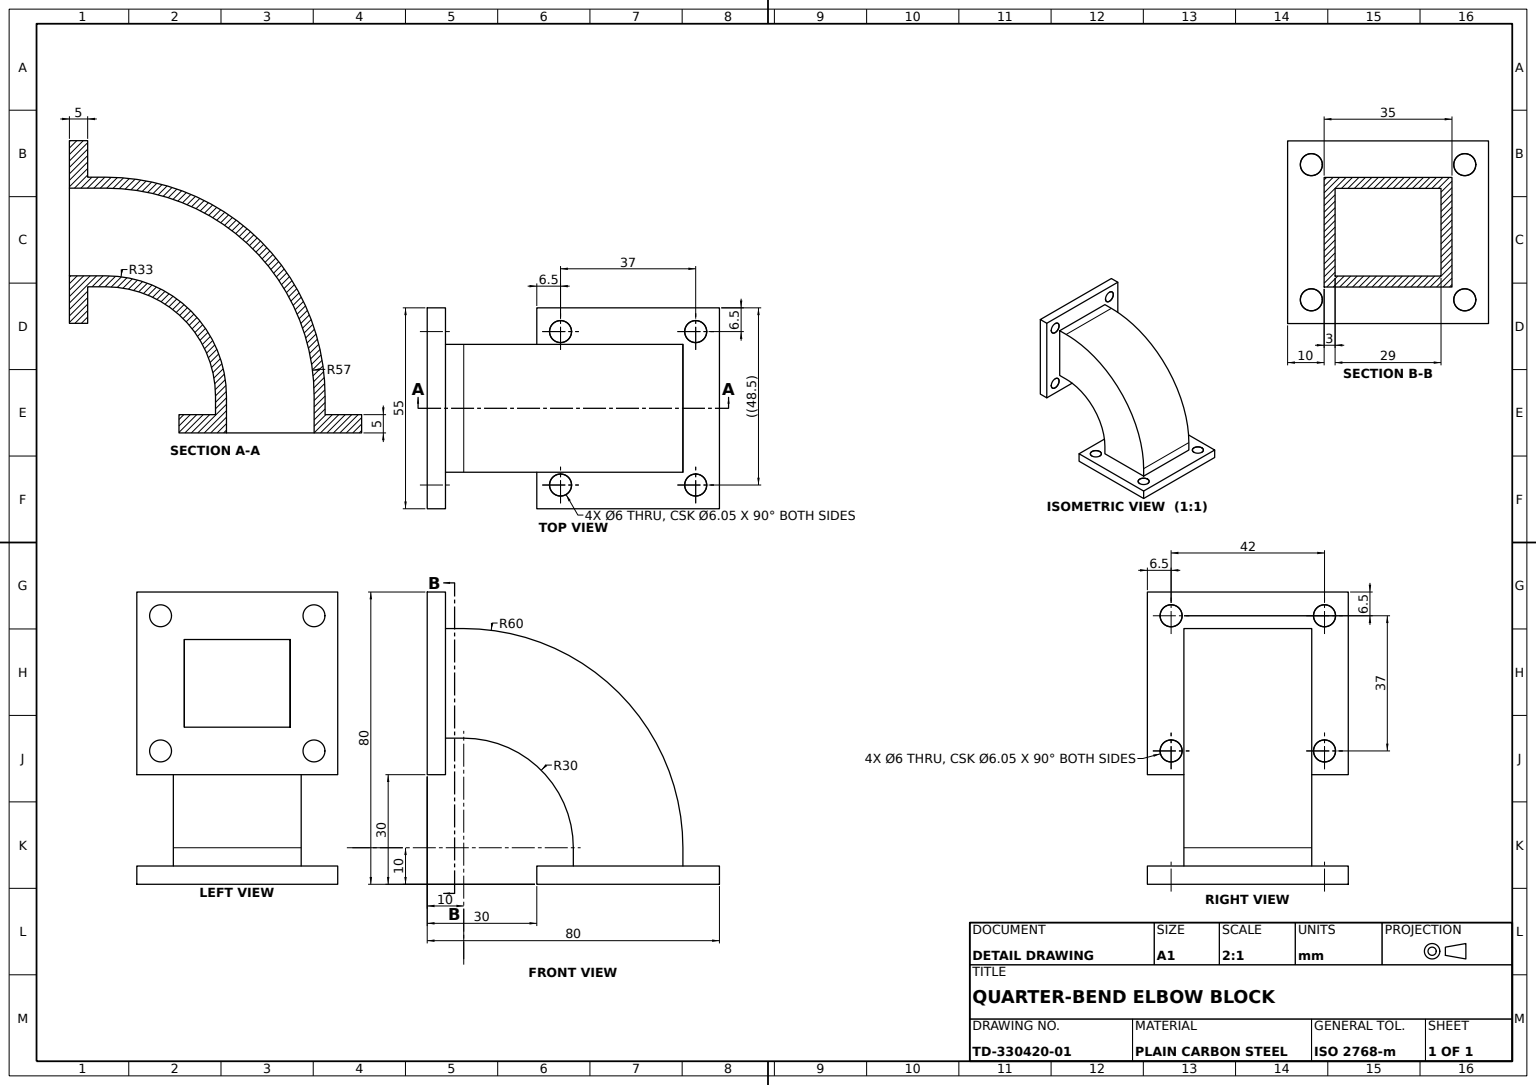
from build123d import *

# Parameters (mm, degrees)
CURVED_DUCT_BODY_DEPTH             = 17.5
SKETCH1_4_W                        = 50
SKETCH1_4_H                        = 5
SKETCH1_4_W_2                      = 5
SKETCH1_4_H_2                      = 50
MOUNTING_FLANGES_DEPTH             = 27.5
SKETCH1_5_W                        = 24
SKETCH1_5_H                        = 5
SKETCH1_5_W_2                      = 5
SKETCH1_5_H_2                      = 24
DUCT_RELIEF_CUT_29MM_DEPTH         = 14.5
DOWEL_HOLES_6_FLANGE_A_D           = 6
DOWEL_HOLES_6_FLANGE_A_CSINK_D     = 6.05
DOWEL_HOLES_6_FLANGE_A_CSINK_ANGLE = 90
DOWEL_HOLES_6_FLANGE_B_D           = 6
DOWEL_HOLES_6_FLANGE_B_CSINK_D     = 6.05
DOWEL_HOLES_6_FLANGE_B_CSINK_ANGLE = 90


with BuildPart() as part:
    # Bracket Profile Sketch → Curved Duct Body (new, symmetric)
    with BuildSketch(Plane.YX):
        with BuildLine():
            Line((15, 5), (15, 10))
            ThreePointArc((15, 10), (-2.573593129, 52.426406871), (-45, 70))
            Line((-45, 70), (-50, 70))
            Line((-50, 70), (-50, 40))
            Line((-50, 40), (-45, 40))
            ThreePointArc((-45, 40), (-23.786796564, 31.213203436), (-15, 10))
            Line((-15, 10), (-15, 5))
            Line((-15, 5), (15, 5))
        make_face()
    extrude(amount=CURVED_DUCT_BODY_DEPTH, both=True)

    # Sketch1_4 → Mounting Flanges (add, symmetric)
    with BuildSketch(Plane.YX):
        with Locations((0, 2.5)):
            Rectangle(SKETCH1_4_W, SKETCH1_4_H)
        with Locations((-52.5, 55)):
            Rectangle(SKETCH1_4_W_2, SKETCH1_4_H_2)
    extrude(amount=MOUNTING_FLANGES_DEPTH, both=True)

    # Sketch1_5 → Duct Relief Cut 29mm (cut, symmetric)
    with BuildSketch(Plane.YX):
        with BuildLine():
            Line((-12, 5), (12, 5))
            Line((12, 5), (12, 10))
            ThreePointArc((12, 10), (-4.694913472, 50.305086528), (-45, 67))
            Line((-45, 67), (-50, 67))
            Line((-50, 67), (-50, 43))
            Line((-50, 43), (-45, 43))
            ThreePointArc((-45, 43), (-21.665476221, 33.334523779), (-12, 10))
            Line((-12, 10), (-12, 5))
        make_face()
        with Locations((0, 2.5)):
            Rectangle(SKETCH1_5_W, SKETCH1_5_H)
        with Locations((-52.5, 55)):
            Rectangle(SKETCH1_5_W_2, SKETCH1_5_H_2)
    extrude(amount=DUCT_RELIEF_CUT_29MM_DEPTH, both=True, mode=Mode.SUBTRACT)

    # Dowel Holes _6 Flange A (through all)
    with Locations(Plane(origin=(5, 0, 0), x_dir=(0, 0, -1), z_dir=(1, 0, 0))):
        with Locations((-21, 18.5), (21, 18.5), (21, -18.5), (-21, -18.5)):
            CounterSinkHole(DOWEL_HOLES_6_FLANGE_A_D / 2, DOWEL_HOLES_6_FLANGE_A_CSINK_D / 2, counter_sink_angle=DOWEL_HOLES_6_FLANGE_A_CSINK_ANGLE)

    # Dowel Holes _6 Flange B (through all)
    with Locations(Plane(origin=(0, -50, 0), x_dir=(1, 0, 0), z_dir=(0, 1, 0))):
        with Locations((73.5, 21), (73.5, -21), (36.5, 21), (36.5, -21)):
            CounterSinkHole(DOWEL_HOLES_6_FLANGE_B_D / 2, DOWEL_HOLES_6_FLANGE_B_CSINK_D / 2, counter_sink_angle=DOWEL_HOLES_6_FLANGE_B_CSINK_ANGLE)


solid = part.part
